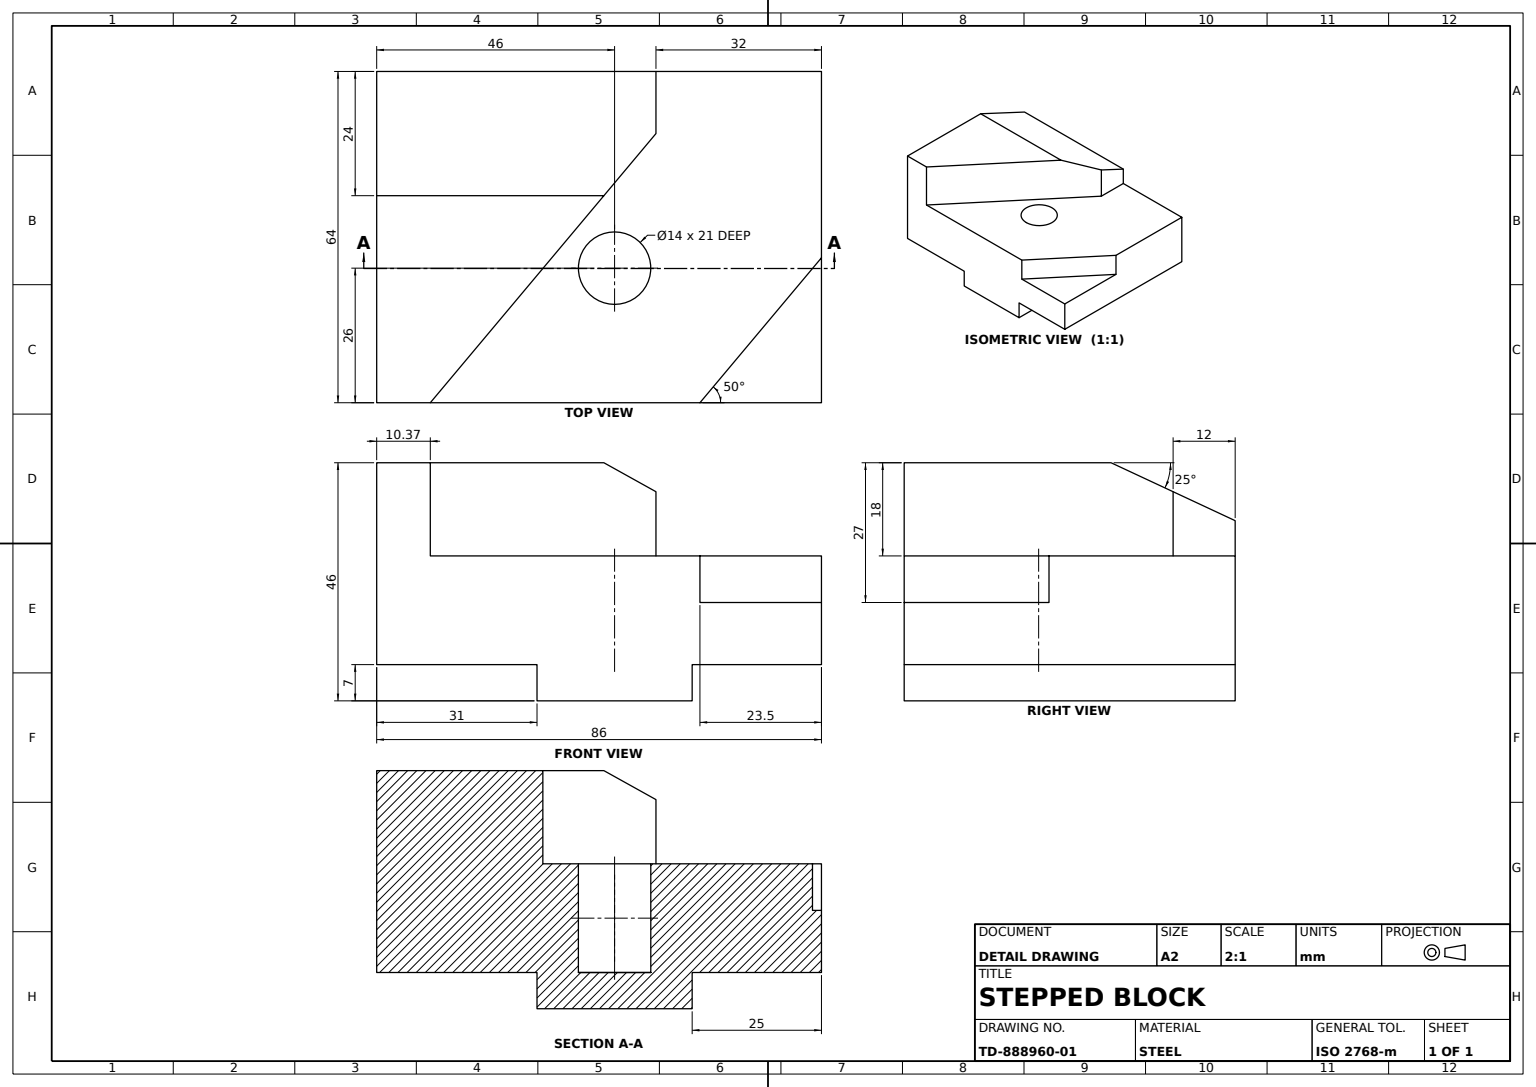
from build123d import *

# Parameters (mm, degrees)
BASE_BLOCK_SKETCH_W         = 86
BASE_BLOCK_SKETCH_H         = 64
BASE_BLOCK_86X64X39_DEPTH   = 39
ANGLED_SIDE_CUT_25DEG_DEPTH = 129
TOP_STEP_CUT_SKETCH_R       = 7
TOP_STEP_CUT_DEPTH          = 18
CORNER_BEVEL_CUT_DEPTH      = 27
THROUGH_HOLE_SKETCH_R       = 7
THROUGH_HOLE_DEPTH          = 97
GUIDE_TONGUE_SKETCH_W       = 30
GUIDE_TONGUE_SKETCH_H       = 7
GUIDE_TONGUE_DEPTH          = 64


with BuildPart() as part:
    # Base Block Sketch → Base Block 86x64x39 (new body)
    with BuildSketch(Plane(origin=(0, 0, 0), x_dir=(1, 0, 0), z_dir=(0, 1, 0))):
        Rectangle(BASE_BLOCK_SKETCH_W, BASE_BLOCK_SKETCH_H)
    extrude(amount=BASE_BLOCK_86X64X39_DEPTH)

    # Angled Side Cut Sketch → Angled Side Cut 25deg (cut)
    with BuildSketch(Plane(origin=(43, 0, 0), x_dir=(0, 0, -1), z_dir=(1, 0, 0))):
        Polygon((8, 39), (32, 27.808616204), (32, 39), align=None)
    extrude(amount=-ANGLED_SIDE_CUT_25DEG_DEPTH, mode=Mode.SUBTRACT)

    # Top Step Cut Sketch → Top Step Cut (cut)
    with BuildSketch(Plane(origin=(0, 39, 0), x_dir=(1, 0, 0), z_dir=(0, 1, 0))):
        Polygon((11, 32), (11, 20), (-32.633180821, -32), (19.502668792, -32), (43, -3.996971117), (43, 32), align=None)
        with Locations(Location((3, -6, 0), (0, 0, 270))):
            Circle(TOP_STEP_CUT_SKETCH_R, mode=Mode.SUBTRACT)
    extrude(amount=-TOP_STEP_CUT_DEPTH, mode=Mode.SUBTRACT)

    # Corner Bevel Cut Sketch → Corner Bevel Cut (cut)
    with BuildSketch(Plane(origin=(0, 39, 0), x_dir=(1, 0, 0), z_dir=(0, 1, 0))):
        Polygon((43, -3.996971117), (19.502668792, -32), (43, -32), align=None)
    extrude(amount=-CORNER_BEVEL_CUT_DEPTH, mode=Mode.SUBTRACT)

    # Through Hole Sketch → Through Hole (cut)
    with BuildSketch(Plane(origin=(0, 39, 0), x_dir=(1, 0, 0), z_dir=(0, 1, 0))):
        with Locations(Location((3, -6, 0), (0, 0, 90))):
            Circle(THROUGH_HOLE_SKETCH_R)
    extrude(amount=-THROUGH_HOLE_DEPTH, mode=Mode.SUBTRACT)

    # Guide Tongue Sketch → Guide Tongue (add)
    with BuildSketch(Plane.XY.offset(32)):
        with Locations((3, -3.5)):
            Rectangle(GUIDE_TONGUE_SKETCH_W, GUIDE_TONGUE_SKETCH_H)
    extrude(amount=-GUIDE_TONGUE_DEPTH)


solid = part.part
